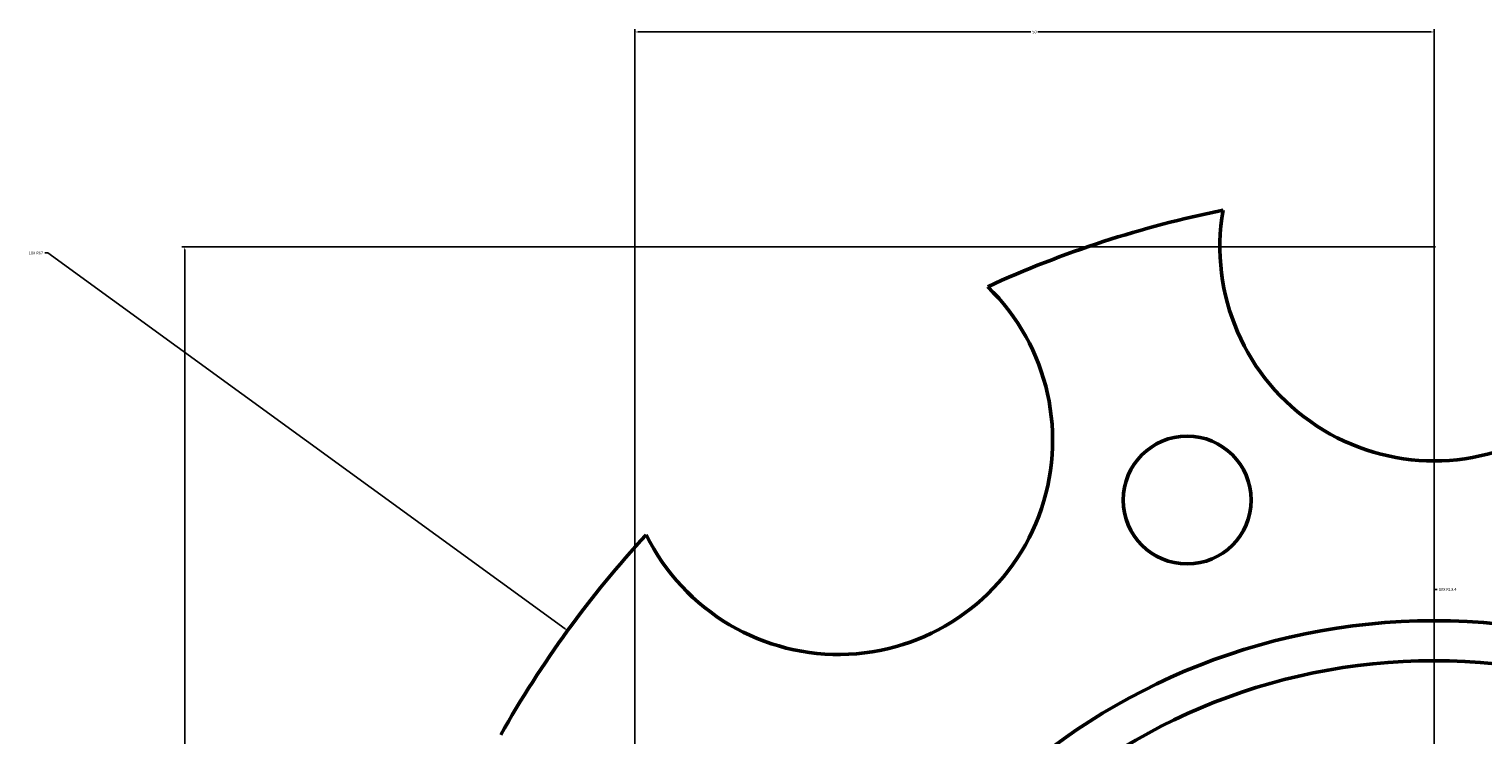
# Model space of a CAD drawing. Units: inches. Extents: x -62 to 104, y -63 to 91.
# Tile 3 of 4: x -62 to 29, y 47 to 91. Entities that reach past the tile are written whole.
import ezdxf

# ---------------------------------------------------------------- set-up
doc = ezdxf.new("R2010")
doc.units = ezdxf.units.IN
doc.header["$MEASUREMENT"] = 0
doc.layers.add('M-DIMS', color=2, linetype='Continuous', lineweight=18)
doc.layers.add('M-OUTL', color=7, linetype='Continuous', lineweight=50)
doc.styles.get("Standard").update_dxf_attribs({"font": 'arial.ttf'})
doc.dimstyles.get("Standard").update_dxf_attribs({"dimtxt": 0.18, "dimasz": 0.18, "dimexe": 0.18, "dimexo": 0.0625, "dimgap": 0.09, "dimtad": 0, "dimtih": 1, "dimtoh": 1, "dimdec": 4, "dimzin": 0, "dimdsep": 46, "dimtxsty": 'Standard', "dimcen": 0.09, "dimadec": 0, "dimazin": 0, "dimtfac": 1, "dimtdec": 4, "dimtofl": 0, "dimtmove": 0, "dimatfit": 3, "dimfxl": 1, "dimtolj": 1, "dimtzin": 0, "dimarcsym": 0})

# ---------------------------------------------------------------- blocks, each defined once
blk = doc.blocks.new('BOLT-HOLE-D8')
blk.add_circle((4, 4), 4)
blk = doc.blocks.new('*D4')
at = {"layer": 'Defpoints', "color": 0, "transparency": 16777216}
for p in [(25.452, 90.58), (-24.548, 13.739), (25.452, 13.739)]:
    blk.add_point(p, dxfattribs=at)
at = {"layer": 'M-DIMS', "color": 0, "lineweight": -2, "transparency": 16777216}
for p, q in [((-24.548, 13.802), (-24.548, 90.76)), ((-24.368, 90.58), (0.233, 90.58)), ((25.272, 90.58), (0.671, 90.58)), ((25.452, 13.802), (25.452, 90.76))]:
    blk.add_line(p, q, dxfattribs=at)
at = {"layer": 'M-DIMS', "color": 0, "transparency": 16777216}
for points in [[(-24.368, 90.61), (-24.368, 90.55), (-24.548, 90.58)], [(25.272, 90.61), (25.272, 90.55), (25.452, 90.58)]]:
    blk.add_solid(points, dxfattribs=at)
at = {"layer": 'M-DIMS', "color": 0, "transparency": 16777216, "insert": (0.452, 90.58), "char_height": 0.18, "attachment_point": 5}
blk.add_mtext('\\A1;50', dxfattribs=at)
blk = doc.blocks.new('*D5')
at = {"layer": 'Defpoints', "color": 0, "transparency": 16777216}
for p in [(-52.703, 77.139), (25.452, 77.139), (25.452, 13.739)]:
    blk.add_point(p, dxfattribs=at)
at = {"layer": 'M-DIMS', "color": 0, "lineweight": -2, "transparency": 16777216}
for p, q in [((25.389, 77.139), (-52.883, 77.139)), ((-52.703, 76.959), (-52.703, 45.621)), ((-52.703, 13.919), (-52.703, 45.257)), ((25.389, 13.739), (-52.883, 13.739))]:
    blk.add_line(p, q, dxfattribs=at)
at = {"layer": 'M-DIMS', "color": 0, "transparency": 16777216}
for points in [[(-52.733, 76.959), (-52.673, 76.959), (-52.703, 77.139)], [(-52.733, 13.919), (-52.673, 13.919), (-52.703, 13.739)]]:
    blk.add_solid(points, dxfattribs=at)
at = {"layer": 'M-DIMS', "color": 0, "transparency": 16777216, "insert": (-52.703, 45.439), "char_height": 0.18, "attachment_point": 5}
blk.add_mtext('\\A1;63.4', dxfattribs=at)
blk = doc.blocks.new('*D6')
at = {"layer": 'Defpoints', "color": 0, "transparency": 16777216}
for p in [(-28.752, 53.121), (25.452, 13.739)]:
    blk.add_point(p, dxfattribs=at)
at = {"layer": 'M-DIMS', "color": 0, "lineweight": -2, "transparency": 16777216}
for p, q in [((-61.454, 76.75), (-61.274, 76.75)), ((-61.274, 76.75), (-28.898, 53.227)), ((25.362, 13.739), (25.542, 13.739)), ((25.452, 13.649), (25.452, 13.829))]:
    blk.add_line(p, q, dxfattribs=at)
at = {"layer": 'M-DIMS', "color": 0, "transparency": 16777216}
blk.add_solid([(-28.88, 53.251), (-28.915, 53.203), (-28.752, 53.121)], dxfattribs=at)
at = {"layer": 'M-DIMS', "color": 0, "transparency": 16777216, "insert": (-62.014, 76.75), "char_height": 0.18, "attachment_point": 5}
blk.add_mtext('\\A1;10X R67', dxfattribs=at)
blk = doc.blocks.new('*D7')
at = {"layer": 'Defpoints', "color": 0, "transparency": 16777216}
for p in [(25.452, 77.139), (25.452, 63.739)]:
    blk.add_point(p, dxfattribs=at)
at = {"layer": 'M-DIMS', "color": 0, "lineweight": -2, "transparency": 16777216}
for p, q in [((25.362, 77.139), (25.542, 77.139)), ((25.452, 77.049), (25.452, 77.229)), ((25.452, 55.699), (25.452, 63.559)), ((25.632, 55.699), (25.452, 55.699))]:
    blk.add_line(p, q, dxfattribs=at)
at = {"layer": 'M-DIMS', "color": 0, "transparency": 16777216}
blk.add_solid([(25.482, 63.559), (25.422, 63.559), (25.452, 63.739)], dxfattribs=at)
at = {"layer": 'M-DIMS', "color": 0, "transparency": 16777216, "insert": (26.296, 55.699), "char_height": 0.18, "attachment_point": 5}
blk.add_mtext('\\A1;10X R13.4', dxfattribs=at)

msp = doc.modelspace()

# ---------------------------------------------------------------- linework, layer by layer
at = {"layer": 'M-OUTL'}
for radius in [40, 37.5]:
    msp.add_circle((25.452, 13.739), radius, dxfattribs=at)
for centre, radius, start, end in [((25.452, 13.739), 67, 101.36555, 114.63445), ((25.452, 77.139), 13.4, 170.17695, 9.82305), ((-11.814, 65.031), 13.4, 206.17695, 45.82305), ((25.452, 13.739), 67, 137.36555, 150.63445)]:
    msp.add_arc(centre, radius, start, end, dxfattribs=at)

# ---------------------------------------------------------------- block references
msp.add_blockref('BOLT-HOLE-D8', (6.001, 57.292), dxfattribs=at)

# ---------------------------------------------------------------- dimensions: what is measured, and where the dimension line sits
at = {"layer": 'M-DIMS'}
dim = msp.add_linear_dim(base=(25.452, 90.58), p1=(-24.548, 13.739), p2=(25.452, 13.739), dimstyle='Standard', override={"dimdec": 0, "dimlfac": 1, "dimrnd": 0, "dimzin": 0, "dimdsep": 46, "dimlunit": 2}, dxfattribs=at)
dim.commit()
dim.dimension.update_dxf_attribs({"geometry": '*D4', "text_midpoint": (0.452, 90.58)})
for center, mpoint, override, picture, middle in [((25.452, 13.739), (-28.752, 53.121), {"dimdec": 0, "dimlfac": 1, "dimrnd": 0, "dimzin": 0, "dimdsep": 46, "dimlunit": 2}, '*D6', (-62.014, 76.75)), ((25.452, 77.139), (25.452, 63.739), {"dimdec": 1, "dimlfac": 1, "dimrnd": 0, "dimzin": 0, "dimdsep": 46, "dimlunit": 2}, '*D7', (26.296, 55.699))]:
    dim = msp.add_radius_dim(center=center, mpoint=mpoint, text='10X <>', dimstyle='Standard', override=override, dxfattribs=at)
    dim.commit()
    dim.dimension.update_dxf_attribs({"geometry": picture, "text_midpoint": middle, "dimtype": 164})
dim = msp.add_linear_dim(base=(-52.703, 77.139), p1=(25.452, 13.739), p2=(25.452, 77.139), angle=90, dimstyle='Standard', override={"dimdec": 1, "dimlfac": 1, "dimrnd": 0, "dimzin": 0, "dimdsep": 46, "dimlunit": 2}, dxfattribs=at)
dim.commit()
dim.dimension.update_dxf_attribs({"geometry": '*D5', "text_midpoint": (-52.703, 45.439)})

doc.saveas('drawing.dxf')
